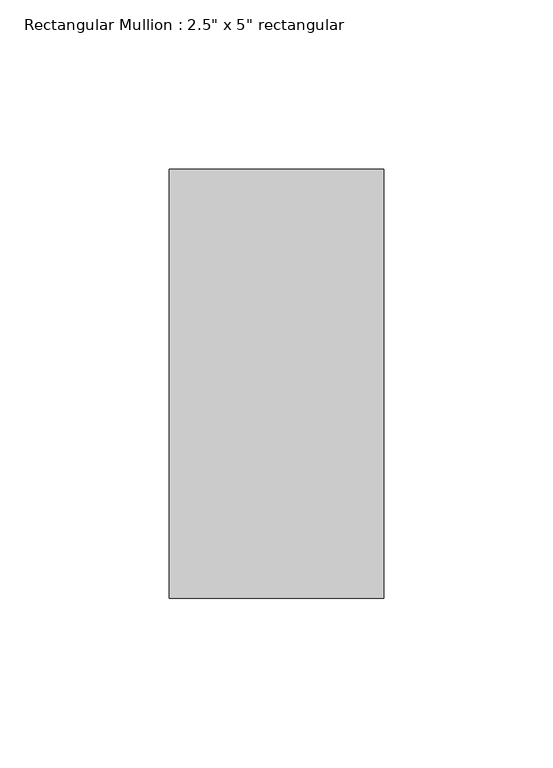
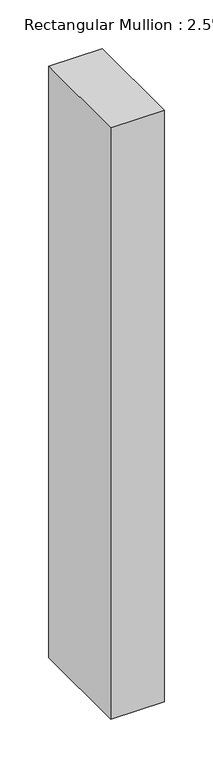
"""IFC4 building model written with IfcOpenShell, lengths in millimetres: member geometry."""

from ifc_helpers import new_model, si_unit, frame, origin, place, context, project, spatial, polyline, outline, extrude, source, transform, mapped, element, save


def member_46fef415(model_context):
    return source(origin(), model_context, "Body", "SweptSolid", [
        extrude(outline(polyline([(31.75, 63.5), (31.75, -63.5), (-31.75, -63.5), (-31.75, 63.5), (31.75, 63.5)])), frame((0.0, 0.0, -740.8042001), z_axis=(0.0, 0.0, 1.0), x_axis=(1.0, 0.0, 0.0)), (0.0, 0.0, 1.0), 740.8042001),
    ])


if __name__ == "__main__":
    model = new_model("IFC4")
    model_context = context("Model", 3, world=origin())
    ifc_project = project(units=[si_unit("LENGTHUNIT", "METRE", prefix="MILLI")], contexts=[model_context])
    site = spatial("IfcSite", under=ifc_project)
    building = spatial("IfcBuilding", under=site)
    placement = place(None, origin())
    member_shape = member_46fef415(model_context)
    element("IfcMember", 1, ObjectType="Rectangular Mullion : 2.5\" x 5\" rectangular", at=placement, inside=building, context=model_context, shape_type="MappedRepresentation", body=[
        mapped(member_shape, transform((0.0, 0.0, 0.0), x_axis=(1.0, 0.0, 0.0), y_axis=(0.0, 1.0, 0.0), z_axis=(0.0, 0.0, 1.0))),
    ])
    save(model, "model.ifc")

# Revit data of these elements
# Type "Rectangular Mullion : 2.5\" x 5\" rectangular"
#   built-in parameter 1007304 = 0.416667 (stored number, unit not read)
#   built-in parameter 1007301 = 0.104167 (stored number, unit not read)
#   built-in parameter 1007300 = 0.104167 (stored number, unit not read)
# Element 1 (IfcMember, "Rectangular Mullion : 2.5\" x 5\" rectangular")
#   Materials on its faces: "Aluminum"
# Materials
#   "Aluminum": class "Metal", colour RGB 247 247 247, transparency 0, Description = "Aluminum 6061", Cost = 0
